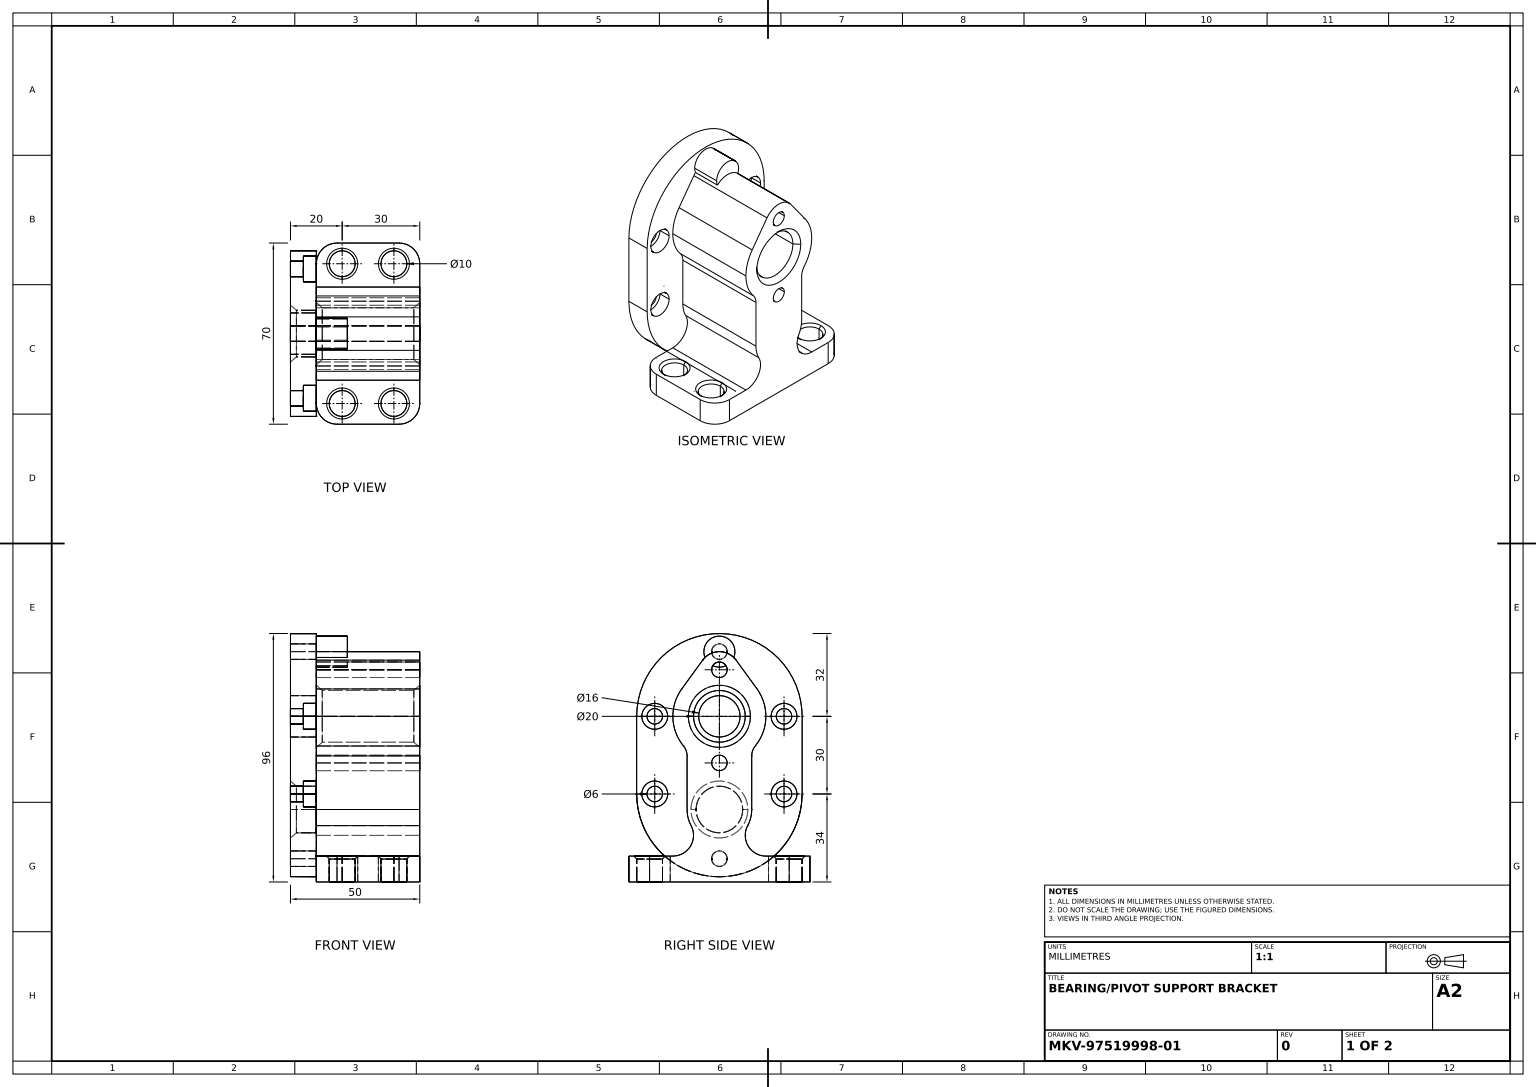
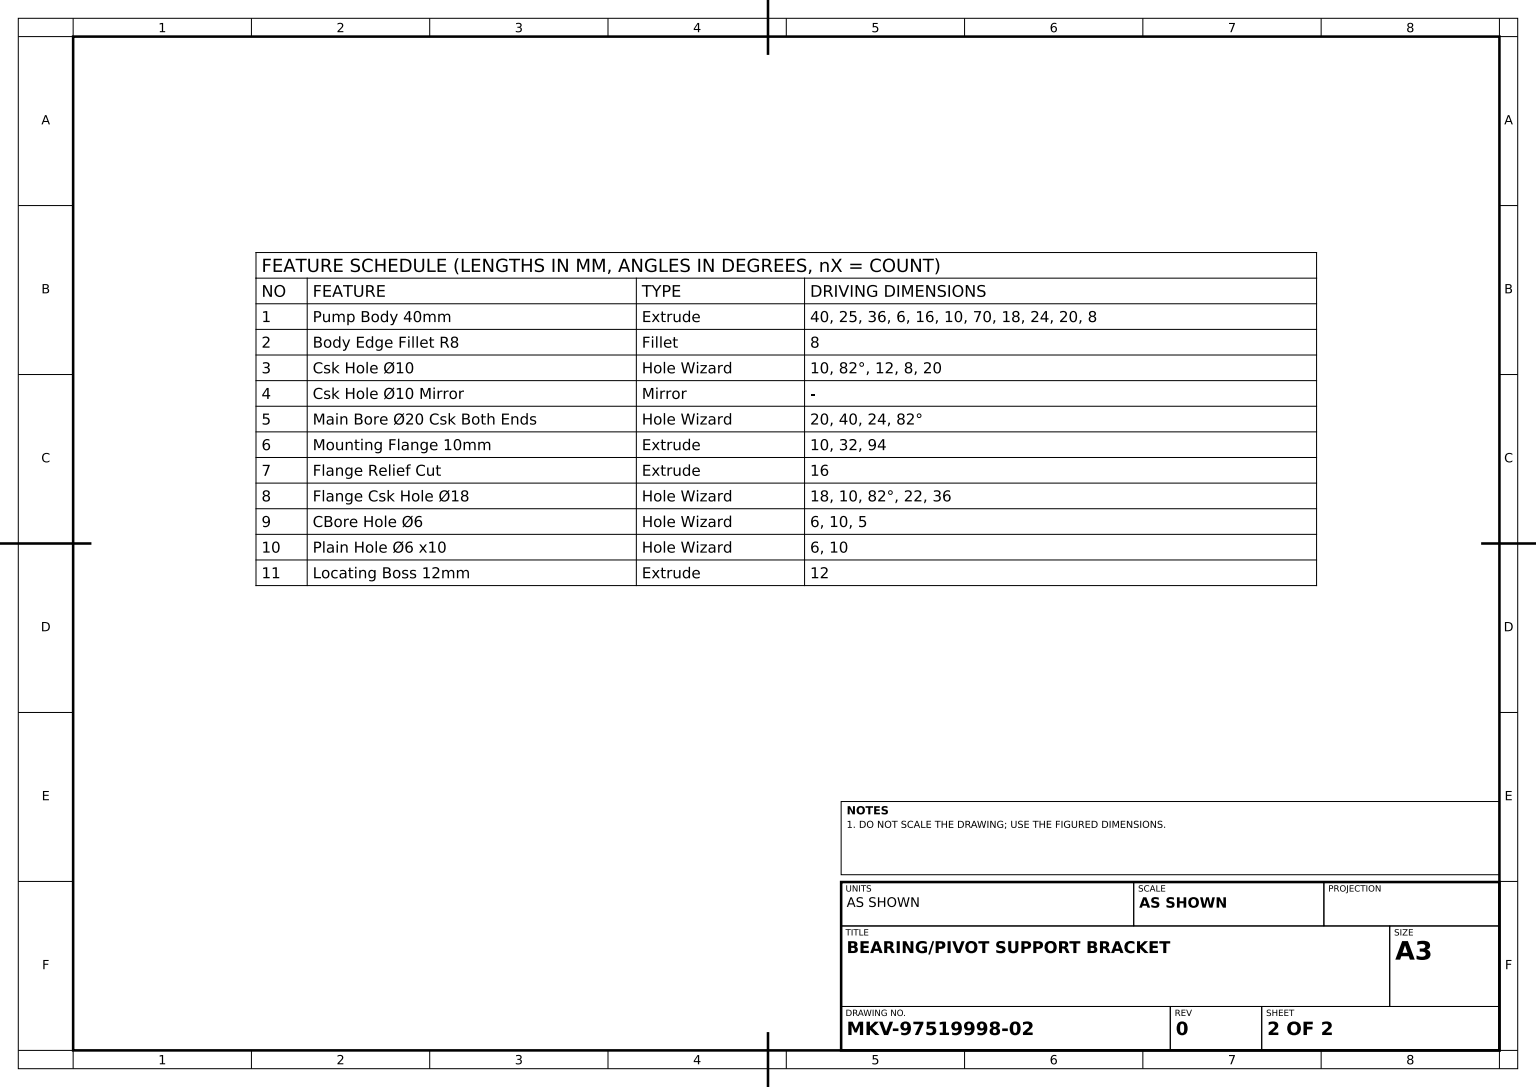
from build123d import *

# Parameters (mm, degrees)
BODY_PROFILE_SKETCH_R       = 3
PUMP_BODY_40MM_DEPTH        = 40
BODY_EDGE_FILLET_R8_R       = 8
CSK_HOLE_10_D               = 10
CSK_HOLE_10_CSINK_D         = 12
CSK_HOLE_10_CSINK_ANGLE     = 82
MOUNTING_FLANGE_10MM_DEPTH  = 10
FLANGE_RELIEF_CUT_REACH     = 90.436
FLANGE_RELIEF_CUT_SKETCH_R  = 8
CBORE_HOLE_6_D              = 6
CBORE_HOLE_6_CBORE_D        = 10
CBORE_HOLE_6_CBORE_DEPTH    = 5
SKETCH16_W                  = 3
SKETCH16_H                  = 10
PLAIN_HOLE_6_X10_AT_2_COUNT = 2
PLAIN_HOLE_6_X10_AT_2_PITCH = 80
LOCATING_BOSS_SKETCH_R      = 6
LOCATING_BOSS_12MM_DEPTH    = 12


with BuildPart() as part:
    # Body Profile Sketch → Pump Body 40mm (new body)
    with BuildSketch(Plane(origin=(0, 0, 0), x_dir=(0, 0, -1), z_dir=(1, 0, 0))):
        with BuildLine():
            Line((-12.5, -15.288884851), (-12.5, -36))
            ThreePointArc((-12.5, -36), (-12.104388127, -39.213597032), (-10.941176471, -42.235294118))
            ThreePointArc((-10.941176471, -42.235294118), (-11.140056594, -50.115966043), (-18, -54))
            Line((-18, -54), (-35, -54))
            Line((-35, -54), (-35, -64))
            Line((-35, -64), (35, -64))
            Line((35, -64), (35, -54))
            Line((35, -54), (18, -54))
            ThreePointArc((18, -54), (11.140056594, -50.115966043), (10.941176471, -42.235294118))
            ThreePointArc((10.941176471, -42.235294118), (12.104388127, -39.213597032), (12.5, -36))
            Line((12.5, -36), (12.5, -15.288884851))
            ThreePointArc((12.5, -15.288884851), (12.854205105, -13.25787525), (13.875, -11.466663639))
            ThreePointArc((13.875, -11.466663639), (17.99141486, -0.555869896), (14.556416913, 10.588235294))
            Line((14.556416913, 10.588235294), (6.469518628, 21.705882353))
            ThreePointArc((6.469518628, 21.705882353), (0, 25), (-6.469518628, 21.705882353))
            Line((-6.469518628, 21.705882353), (-14.556416913, 10.588235294))
            ThreePointArc((-14.556416913, 10.588235294), (-17.99141486, -0.555869896), (-13.875, -11.466663639))
            ThreePointArc((-13.875, -11.466663639), (-12.854205105, -13.25787525), (-12.5, -15.288884851))
        make_face()
        with Locations((0, -18)):
            Circle(BODY_PROFILE_SKETCH_R, mode=Mode.SUBTRACT)
        with Locations((0, 18)):
            Circle(BODY_PROFILE_SKETCH_R, mode=Mode.SUBTRACT)
    extrude(amount=PUMP_BODY_40MM_DEPTH)

    # Body Edge Fillet R8
    body_edge_fillet_r8_edges = [part.edges().sort_by_distance(p)[0] for p in [
        (0, -59, -35),
        (0, -59, 35),
        (40, -59, 35),
        (40, -59, -35),
    ]]
    fillet(body_edge_fillet_r8_edges, radius=BODY_EDGE_FILLET_R8_R)

    # Csk Hole Ø10 (through all)
    with Locations(Plane(origin=(10, -54, 27), x_dir=(0, 0, 1), z_dir=(0, 1, 0))):
        with Locations((0, 0), (0, 20)):
            csk_hole_10 = CounterSinkHole(CSK_HOLE_10_D / 2, CSK_HOLE_10_CSINK_D / 2, counter_sink_angle=CSK_HOLE_10_CSINK_ANGLE)

    # Csk Hole Ø10 Mirror: Csk Hole Ø10 across plane
    add(csk_hole_10.mirror(Plane.XY), mode=Mode.SUBTRACT)

    # Sketch7 → Main Bore Ø20 Csk Both Ends (revolve, cut)
    with BuildSketch(Plane(origin=(40, 0, 0), x_dir=(0, 0, -1), z_dir=(0, 1, 0))):
        Polygon((0, 0), (0, 40), (12, 40), (10, 37.699263186), (10, 2.300736814), (12, 0), align=None)
    revolve(axis=Axis((46.35, 0, 0), (-1, 0, 0)), mode=Mode.SUBTRACT)

    # Mounting Flange Sketch → Mounting Flange 10mm (add)
    with BuildSketch(Plane.ZY):
        with BuildLine():
            Line((32, 0), (32, -30))
            ThreePointArc((32, -30), (0, -62), (-32, -30))
            Line((-32, -30), (-32, 0))
            ThreePointArc((-32, 0), (0, 32), (32, 0))
        make_face()
    extrude(amount=MOUNTING_FLANGE_10MM_DEPTH)

    # Flange Relief Cut Sketch → Flange Relief Cut (cut, up to next)
    with BuildSketch(Plane.ZY.offset(10), mode=Mode.PRIVATE) as flange_relief_cut_sk1:
        Circle(FLANGE_RELIEF_CUT_SKETCH_R)
    flange_relief_cut_tool1 = extrude(flange_relief_cut_sk1.sketch, amount=-FLANGE_RELIEF_CUT_REACH, mode=Mode.PRIVATE) & part.part
    add(flange_relief_cut_tool1.solids().sort_by_distance((-10, 0, 0))[0], mode=Mode.SUBTRACT)

    # Sketch9 → Flange Csk Hole Ø18 (revolve, cut)
    with BuildSketch(Plane(origin=(-10, -36, 0), x_dir=(0, 0, 1), z_dir=(0, 1, 0))):
        Polygon((0, 0), (0, 9.797958971), (9, 9.797958971), (9, 2.300736814), (11, 0), align=None)
    revolve(axis=Axis((-16.445314094, -36, 0), (1, 0, 0)), mode=Mode.SUBTRACT)

    # CBore Hole Ø6 (through all)
    with Locations(Plane(origin=(0, -30, -25), x_dir=(0, 0, 1), z_dir=(1, 0, 0))):
        with Locations((0, 0), (0, -30), (50, 0), (50, -30)):
            CounterBoreHole(CBORE_HOLE_6_D / 2, CBORE_HOLE_6_CBORE_D / 2, CBORE_HOLE_6_CBORE_DEPTH)

    # Sketch16 → Plain Hole Ø6 x10 (revolve, cut)
    with BuildSketch(Plane(origin=(0, -55, 0), x_dir=(0, 0, -1), z_dir=(0, 1, 0))):
        with Locations((1.5, 5)):
            Rectangle(SKETCH16_W, SKETCH16_H)
    plain_hole_6_x10 = revolve(axis=Axis((-110, -55, 0), (1, 0, 0)), mode=Mode.SUBTRACT)

    # Plain Hole Ø6 x10 at 2: Plain Hole Ø6 x10 ×2
    with Locations(*[(0, i * PLAIN_HOLE_6_X10_AT_2_PITCH, 0) for i in range(1, PLAIN_HOLE_6_X10_AT_2_COUNT)]):
        add(plain_hole_6_x10, mode=Mode.SUBTRACT)

    # Locating Boss Sketch → Locating Boss 12mm (add)
    with BuildSketch(Plane(origin=(0, 0, 0), x_dir=(0, 0, -1), z_dir=(1, 0, 0))):
        with Locations((0, 25)):
            Circle(LOCATING_BOSS_SKETCH_R)
    extrude(amount=LOCATING_BOSS_12MM_DEPTH)


solid = part.part
